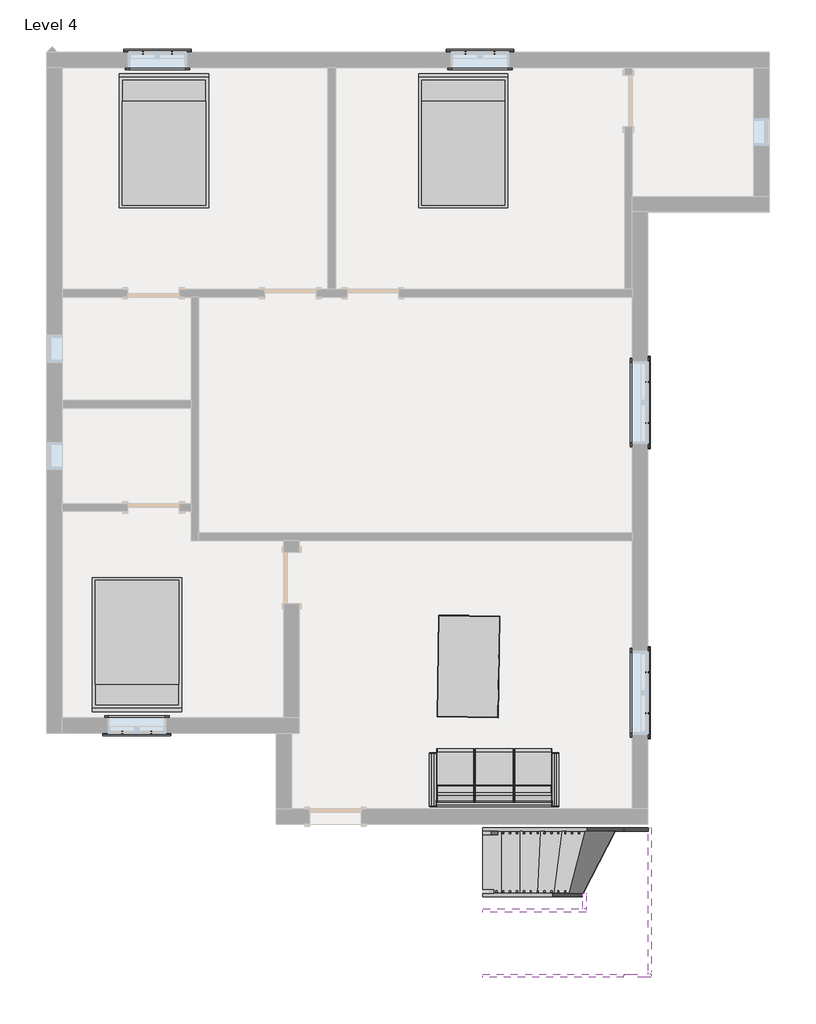
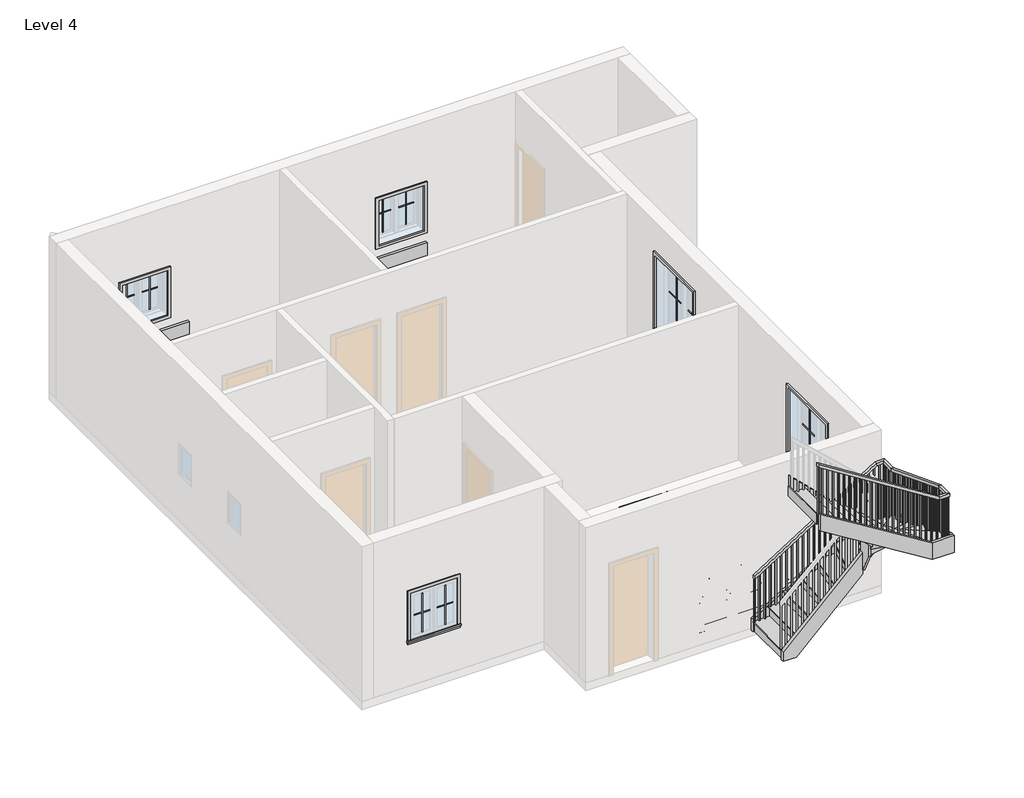
# One storey, part 2 of 2: 20 proxies, 8 members, 5 furniture elements, 1 railing, 1 stair flight.
"""IFC4 building model written with IfcOpenShell, lengths in millimetres."""

from ifc_helpers import new_model, si_unit, frame, origin, place, context, project, spatial, polyline, outline, extrude, faceted_brep, transform, mapped, element, save
from components import muntin_pattern_2x2_muntin_pattern_2x2_b3fe6957, muntin_pattern_2x2_muntin_pattern_2x2_3e0ecaf2, muntin_pattern_2x2_muntin_pattern_2x2_6dad3731, muntin_pattern_2x2_muntin_pattern_2x2_a30a3345, trim_window_exterior_flat_with_sill_41619996, trim_window_exterior_flat_with_sill_92b9b949, trim_window_interior_flat_picture_frame_51c85655, trim_window_interior_flat_picture_frame_3bb882cf, furniture_2fc85b74, furniture_29a9adb8, furniture_57072a26, bed_17739_bed_17739_15c61121, dining_table_14755_dining_table_14755_d89cb775, stair_flight_27d53fa0

model = new_model("IFC4")

# Units and contexts
model_context = context("Model", 3, world=origin())
ifc_project = project(units=[si_unit("LENGTHUNIT", "METRE", prefix="MILLI")], contexts=[model_context])

# Site, building, storey
site = spatial("IfcSite", under=ifc_project)
building = spatial("IfcBuilding", under=site)
storey = spatial("IfcBuildingStorey", under=building, Name="Level 4", Elevation=6400.8)

# Proxies
placement = place(None, origin())
muntin_pattern_2x2_muntin_pattern_2x2_shape = muntin_pattern_2x2_muntin_pattern_2x2_b3fe6957(model_context)
element("IfcBuildingElementProxy", 1, Name="Muntin Pattern_2x2 : Muntin Pattern_2x2", ObjectType="Muntin Pattern_2x2 : Muntin Pattern_2x2", at=placement, inside=storey, context=model_context, shape_type="MappedRepresentation", body=[
    mapped(muntin_pattern_2x2_muntin_pattern_2x2_shape, transform((-4708.0540084, 8034.3685985, 7385.05), x_axis=(1.0, 0.0, 0.0), y_axis=(0.0, 1.0, 0.0), z_axis=(0.0, 0.0, 1.0))),
])
element("IfcBuildingElementProxy", 2, Name="Muntin Pattern_2x2 : Muntin Pattern_2x2", ObjectType="Muntin Pattern_2x2 : Muntin Pattern_2x2", at=placement, inside=storey, context=model_context, shape_type="MappedRepresentation", body=[
    mapped(muntin_pattern_2x2_muntin_pattern_2x2_shape, transform((54.4459916, 8034.3685985, 7385.05), x_axis=(1.0, 0.0, 0.0), y_axis=(0.0, 1.0, 0.0), z_axis=(0.0, 0.0, 1.0))),
])
element("IfcBuildingElementProxy", 3, Name="Muntin Pattern_2x2 : Muntin Pattern_2x2", ObjectType="Muntin Pattern_2x2 : Muntin Pattern_2x2", at=placement, inside=storey, context=model_context, shape_type="MappedRepresentation", body=[
    mapped(muntin_pattern_2x2_muntin_pattern_2x2_shape, transform((-4584.2290084, -2004.9814015, 7385.05), x_axis=(-1.0, 0.0, 0.0), y_axis=(0.0, -1.0, 0.0), z_axis=(0.0, 0.0, 1.0))),
])
muntin_pattern_2x2_muntin_pattern_2x2_2_shape = muntin_pattern_2x2_muntin_pattern_2x2_3e0ecaf2(model_context)
element("IfcBuildingElementProxy", 4, Name="Muntin Pattern_2x2 : Muntin Pattern_2x2", ObjectType="Muntin Pattern_2x2 : Muntin Pattern_2x2", at=placement, inside=storey, context=model_context, shape_type="MappedRepresentation", body=[
    mapped(muntin_pattern_2x2_muntin_pattern_2x2_2_shape, transform((-4279.4290084, 8034.3685985, 7385.05), x_axis=(-1.0, 0.0, 0.0), y_axis=(0.0, -1.0, 0.0), z_axis=(0.0, 0.0, 1.0))),
])
element("IfcBuildingElementProxy", 5, Name="Muntin Pattern_2x2 : Muntin Pattern_2x2", ObjectType="Muntin Pattern_2x2 : Muntin Pattern_2x2", at=placement, inside=storey, context=model_context, shape_type="MappedRepresentation", body=[
    mapped(muntin_pattern_2x2_muntin_pattern_2x2_2_shape, transform((483.0709916, 8034.3685985, 7385.05), x_axis=(-1.0, 0.0, 0.0), y_axis=(0.0, -1.0, 0.0), z_axis=(0.0, 0.0, 1.0))),
])
element("IfcBuildingElementProxy", 6, Name="Muntin Pattern_2x2 : Muntin Pattern_2x2", ObjectType="Muntin Pattern_2x2 : Muntin Pattern_2x2", at=placement, inside=storey, context=model_context, shape_type="MappedRepresentation", body=[
    mapped(muntin_pattern_2x2_muntin_pattern_2x2_2_shape, transform((-5012.8540084, -2004.9814015, 7385.05), x_axis=(1.0, 0.0, 0.0), y_axis=(0.0, 1.0, 0.0), z_axis=(0.0, 0.0, 1.0))),
])
muntin_pattern_2x2_muntin_pattern_2x2_3_shape = muntin_pattern_2x2_muntin_pattern_2x2_6dad3731(model_context)
element("IfcBuildingElementProxy", 7, Name="Muntin Pattern_2x2 : Muntin Pattern_2x2", ObjectType="Muntin Pattern_2x2 : Muntin Pattern_2x2", at=placement, inside=storey, context=model_context, shape_type="MappedRepresentation", body=[
    mapped(muntin_pattern_2x2_muntin_pattern_2x2_3_shape, transform((2735.7334916, -1114.3939015, 7385.05), x_axis=(0.0, -1.0, 0.0), y_axis=(1.0, 0.0, 0.0), z_axis=(0.0, 0.0, 1.0))),
])
element("IfcBuildingElementProxy", 8, Name="Muntin Pattern_2x2 : Muntin Pattern_2x2", ObjectType="Muntin Pattern_2x2 : Muntin Pattern_2x2", at=placement, inside=storey, context=model_context, shape_type="MappedRepresentation", body=[
    mapped(muntin_pattern_2x2_muntin_pattern_2x2_3_shape, transform((2735.7334916, 3171.8560985, 7385.05), x_axis=(0.0, -1.0, 0.0), y_axis=(1.0, 0.0, 0.0), z_axis=(0.0, 0.0, 1.0))),
])
muntin_pattern_2x2_muntin_pattern_2x2_4_shape = muntin_pattern_2x2_muntin_pattern_2x2_a30a3345(model_context)
element("IfcBuildingElementProxy", 9, Name="Muntin Pattern_2x2 : Muntin Pattern_2x2", ObjectType="Muntin Pattern_2x2 : Muntin Pattern_2x2", at=placement, inside=storey, context=model_context, shape_type="MappedRepresentation", body=[
    mapped(muntin_pattern_2x2_muntin_pattern_2x2_4_shape, transform((2735.7334916, -1720.8189015, 7385.05), x_axis=(0.0, 1.0, 0.0), y_axis=(-1.0, 0.0, 0.0), z_axis=(0.0, 0.0, 1.0))),
])
element("IfcBuildingElementProxy", 10, Name="Muntin Pattern_2x2 : Muntin Pattern_2x2", ObjectType="Muntin Pattern_2x2 : Muntin Pattern_2x2", at=placement, inside=storey, context=model_context, shape_type="MappedRepresentation", body=[
    mapped(muntin_pattern_2x2_muntin_pattern_2x2_4_shape, transform((2735.7334916, 2565.4310985, 7385.05), x_axis=(0.0, 1.0, 0.0), y_axis=(-1.0, 0.0, 0.0), z_axis=(0.0, 0.0, 1.0))),
])
trim_window_exterior_flat_with_sill_shape = trim_window_exterior_flat_with_sill_41619996(model_context)
element("IfcBuildingElementProxy", 11, Name="Trim-Window-Exterior-Flat : with Sill", ObjectType="Trim-Window-Exterior-Flat : with Sill", at=placement, inside=storey, context=model_context, shape_type="MappedRepresentation", body=[
    mapped(trim_window_exterior_flat_with_sill_shape, transform((-4493.7415084, 8043.8935985, 8229.6), x_axis=(-1.0, 0.0, 0.0), y_axis=(0.0, 0.0, 1.0), z_axis=(0.0, 1.0, 0.0))),
])
element("IfcBuildingElementProxy", 12, Name="Trim-Window-Exterior-Flat : with Sill", ObjectType="Trim-Window-Exterior-Flat : with Sill", at=placement, inside=storey, context=model_context, shape_type="MappedRepresentation", body=[
    mapped(trim_window_exterior_flat_with_sill_shape, transform((268.7584916, 8043.8935985, 8229.6), x_axis=(-1.0, 0.0, 0.0), y_axis=(0.0, 0.0, 1.0), z_axis=(0.0, 1.0, 0.0))),
])
element("IfcBuildingElementProxy", 13, Name="Trim-Window-Exterior-Flat : with Sill", ObjectType="Trim-Window-Exterior-Flat : with Sill", at=placement, inside=storey, context=model_context, shape_type="MappedRepresentation", body=[
    mapped(trim_window_exterior_flat_with_sill_shape, transform((-4798.5415084, -2014.5064015, 8229.6), x_axis=(1.0, 0.0, 0.0), y_axis=(0.0, 0.0, 1.0), z_axis=(0.0, -1.0, 0.0))),
])
trim_window_exterior_flat_with_sill_2_shape = trim_window_exterior_flat_with_sill_92b9b949(model_context)
element("IfcBuildingElementProxy", 14, Name="Trim-Window-Exterior-Flat : with Sill", ObjectType="Trim-Window-Exterior-Flat : with Sill", at=placement, inside=storey, context=model_context, shape_type="MappedRepresentation", body=[
    mapped(trim_window_exterior_flat_with_sill_2_shape, transform((2745.2584916, -1417.6064015, 8839.2), x_axis=(0.0, 1.0, 0.0), y_axis=(0.0, 0.0, 1.0), z_axis=(1.0, 0.0, 0.0))),
])
element("IfcBuildingElementProxy", 15, Name="Trim-Window-Exterior-Flat : with Sill", ObjectType="Trim-Window-Exterior-Flat : with Sill", at=placement, inside=storey, context=model_context, shape_type="MappedRepresentation", body=[
    mapped(trim_window_exterior_flat_with_sill_2_shape, transform((2745.2584916, 2868.6435985, 8839.2), x_axis=(0.0, 1.0, 0.0), y_axis=(0.0, 0.0, 1.0), z_axis=(1.0, 0.0, 0.0))),
])
trim_window_interior_flat_picture_frame_shape = trim_window_interior_flat_picture_frame_51c85655(model_context)
element("IfcBuildingElementProxy", 16, Name="Trim-Window-Interior-Flat : Picture Frame", ObjectType="Trim-Window-Interior-Flat : Picture Frame", at=placement, inside=storey, context=model_context, shape_type="MappedRepresentation", body=[
    mapped(trim_window_interior_flat_picture_frame_shape, transform((-4493.7415084, 7815.2935985, 8229.6), x_axis=(1.0, 0.0, 0.0), y_axis=(0.0, 0.0, 1.0), z_axis=(0.0, -1.0, 0.0))),
])
element("IfcBuildingElementProxy", 17, Name="Trim-Window-Interior-Flat : Picture Frame", ObjectType="Trim-Window-Interior-Flat : Picture Frame", at=placement, inside=storey, context=model_context, shape_type="MappedRepresentation", body=[
    mapped(trim_window_interior_flat_picture_frame_shape, transform((268.7584916, 7815.2935985, 8229.6), x_axis=(1.0, 0.0, 0.0), y_axis=(0.0, 0.0, 1.0), z_axis=(0.0, -1.0, 0.0))),
])
element("IfcBuildingElementProxy", 18, Name="Trim-Window-Interior-Flat : Picture Frame", ObjectType="Trim-Window-Interior-Flat : Picture Frame", at=placement, inside=storey, context=model_context, shape_type="MappedRepresentation", body=[
    mapped(trim_window_interior_flat_picture_frame_shape, transform((-4798.5415084, -1785.9064015, 8229.6), x_axis=(-1.0, 0.0, 0.0), y_axis=(0.0, 0.0, 1.0), z_axis=(0.0, 1.0, 0.0))),
])
trim_window_interior_flat_picture_frame_2_shape = trim_window_interior_flat_picture_frame_3bb882cf(model_context)
element("IfcBuildingElementProxy", 19, Name="Trim-Window-Interior-Flat : Picture Frame", ObjectType="Trim-Window-Interior-Flat : Picture Frame", at=placement, inside=storey, context=model_context, shape_type="MappedRepresentation", body=[
    mapped(trim_window_interior_flat_picture_frame_2_shape, transform((2516.6584916, -1417.6064015, 8839.2), x_axis=(0.0, -1.0, 0.0), y_axis=(0.0, 0.0, 1.0), z_axis=(-1.0, 0.0, 0.0))),
])
element("IfcBuildingElementProxy", 20, Name="Trim-Window-Interior-Flat : Picture Frame", ObjectType="Trim-Window-Interior-Flat : Picture Frame", at=placement, inside=storey, context=model_context, shape_type="MappedRepresentation", body=[
    mapped(trim_window_interior_flat_picture_frame_2_shape, transform((2516.6584916, 2868.6435985, 8839.2), x_axis=(0.0, -1.0, 0.0), y_axis=(0.0, 0.0, 1.0), z_axis=(-1.0, 0.0, 0.0))),
])

# Furniture
furniture_shape = furniture_2fc85b74(model_context)
furniture_2_shape = furniture_29a9adb8(model_context)
furniture_3_shape = furniture_57072a26(model_context)
element("IfcFurniture", 21, at=placement, inside=storey, context=model_context, shape_type="MappedRepresentation", body=[
    mapped(furniture_shape, transform((477.9947981, -2301.7922014, 6400.8), x_axis=(-1.0, 0.0, 0.0), y_axis=(0.0, -1.0, 0.0), z_axis=(0.0, 0.0, 1.0))),
    mapped(furniture_2_shape, transform((477.9947981, -2301.7922014, 6400.8), x_axis=(-1.0, 0.0, 0.0), y_axis=(0.0, -1.0, 0.0), z_axis=(0.0, 0.0, 1.0))),
    mapped(furniture_3_shape, transform((477.9947981, -2301.7922014, 6400.8), x_axis=(-1.0, 0.0, 0.0), y_axis=(0.0, -1.0, 0.0), z_axis=(0.0, 0.0, 1.0))),
])
bed_17739_bed_17739_shape = bed_17739_bed_17739_15c61121(model_context)
element("IfcFurniture", 22, ObjectType="Bed_17739 : Bed_17739", at=placement, inside=storey, context=model_context, shape_type="MappedRepresentation", body=[
    mapped(bed_17739_bed_17739_shape, transform((-4398.4915084, 6710.3935985, 6400.8), x_axis=(1.0, 0.0, 0.0), y_axis=(0.0, 1.0, 0.0), z_axis=(0.0, 0.0, 1.0))),
])
element("IfcFurniture", 23, ObjectType="Bed_17739 : Bed_17739", at=placement, inside=storey, context=model_context, shape_type="MappedRepresentation", body=[
    mapped(bed_17739_bed_17739_shape, transform((21.1084916, 6710.3935985, 6400.8), x_axis=(1.0, 0.0, 0.0), y_axis=(0.0, 1.0, 0.0), z_axis=(0.0, 0.0, 1.0))),
])
element("IfcFurniture", 24, ObjectType="Bed_17739 : Bed_17739", at=placement, inside=storey, context=model_context, shape_type="MappedRepresentation", body=[
    mapped(bed_17739_bed_17739_shape, transform((-4798.5415084, -681.0064015, 6400.8), x_axis=(-1.0, 0.0, 0.0), y_axis=(0.0, -1.0, 0.0), z_axis=(0.0, 0.0, 1.0))),
])
dining_table_14755_dining_table_14755_shape = dining_table_14755_dining_table_14755_d89cb775(model_context)
element("IfcFurniture", 25, ObjectType="Dining_table_14755 : Dining_table_14755", at=placement, inside=storey, context=model_context, shape_type="MappedRepresentation", body=[
    mapped(dining_table_14755_dining_table_14755_shape, transform((535.647979, -1785.9064015, 6400.8), x_axis=(0.016088397262737867, 0.9998705733611308, 0.0), y_axis=(-0.9998705733611308, 0.016088397262737867, 0.0), z_axis=(0.0, 0.0, 1.0))),
])

# Members
element("IfcMember", 26, ObjectType="Stringer - 2\" Width", at=placement, inside=storey, context=model_context, shape_type="SweptSolid", body=[
    extrude(outline(polyline([(6644.4922047, 306.9570026), (6400.8, 306.9570026), (6400.8, 492.4029437), (7577.0227917, 2394.3741942), (7935.3990341, 2394.3741942), (6644.4922047, 306.9570026)])), frame((0.0, -3462.3064015, 0.0), z_axis=(0.0, 1.0, 0.0), x_axis=(0.0, 0.0, 1.0)), (0.0, 0.0, 1.0), 50.8),
])
element("IfcMember", 27, ObjectType="Stringer - 2\" Width", at=placement, inside=storey, context=model_context, shape_type="SweptSolid", body=[
    extrude(outline(polyline([(2394.3741942, -3462.3064015), (2394.3741942, -3411.5064015), (2749.0886944, -3411.5064015), (2749.0886944, -3462.3064015), (2394.3741942, -3462.3064015)])), frame((0.0, 0.0, 7577.0227917), z_axis=(0.0, 0.0, 1.0), x_axis=(1.0, 0.0, 0.0)), (0.0, 0.0, 1.0), 358.3762424),
])
element("IfcMember", 28, ObjectType="Stringer - 2\" Width", at=placement, inside=storey, context=model_context, shape_type="SweptSolid", body=[
    extrude(outline(polyline([(-3411.5064015, 7915.8385252), (-3411.5064015, 7630.5990341), (-3601.4476233, 7630.5990341), (-5570.5064015, 8388.7839126), (-5570.5064015, 8729.4251697), (-5524.4474131, 8729.4251697), (-3411.5064015, 7915.8385252)])), frame((2749.0886944, 0.0, 0.0), z_axis=(1.0, 0.0, 0.0), x_axis=(0.0, 1.0, 0.0)), (0.0, 0.0, 1.0), 50.8),
])
element("IfcMember", 29, ObjectType="Stringer - 2\" Width", at=placement, inside=storey, context=model_context, shape_type="SweptSolid", body=[
    extrude(outline(polyline([(2799.8886944, -5570.5064015), (2799.8886944, -5621.3064015), (2394.3741942, -5621.3064015), (2394.3741942, -5570.5064015), (2799.8886944, -5570.5064015)])), frame((0.0, 0.0, 8402.8105246), z_axis=(0.0, 0.0, 1.0), x_axis=(1.0, 0.0, 0.0)), (0.0, 0.0, 1.0), 326.614645),
])
element("IfcMember", 30, ObjectType="Stringer - 2\" Width", at=placement, inside=storey, context=model_context, shape_type="SweptSolid", body=[
    extrude(outline(polyline([(8402.8105246, 2394.3741942), (8729.4251697, 2394.3741942), (10020.3319991, 306.9570026), (9693.7173541, 306.9570026), (8402.8105246, 2394.3741942)])), frame((0.0, -5621.3064015, 0.0), z_axis=(0.0, 1.0, 0.0), x_axis=(0.0, 0.0, 1.0)), (0.0, 0.0, 1.0), 50.8),
])
element("IfcMember", 31, ObjectType="Stringer - 2\" Width", at=placement, inside=storey, context=model_context, shape_type="SweptSolid", body=[
    extrude(outline(polyline([(6586.349344, 306.9570026), (6400.8, 306.9570026), (6400.8, 553.146333), (7605.0088874, 1783.8886944), (8031.4399862, 1783.8886944), (6586.349344, 306.9570026)])), frame((0.0, -4427.5064015, 0.0), z_axis=(0.0, 1.0, 0.0), x_axis=(0.0, 0.0, 1.0)), (0.0, 0.0, 1.0), 50.8),
])
element("IfcMember", 32, ObjectType="Stringer - 2\" Width", at=placement, inside=storey, context=model_context, shape_type="SweptSolid", body=[
    extrude(outline(polyline([(-4376.7064015, 8276.0734955), (-4376.7064015, 7654.7136944), (-4412.6455235, 7654.7136944), (-4605.3064015, 8049.5203552), (-4605.3064015, 8686.3067712), (-4576.8952811, 8686.3067712), (-4376.7064015, 8276.0734955)])), frame((1783.8886944, 0.0, 0.0), z_axis=(1.0, 0.0, 0.0), x_axis=(0.0, 1.0, 0.0)), (0.0, 0.0, 1.0), 50.8),
])
element("IfcMember", 33, ObjectType="Stringer - 2\" Width", at=placement, inside=storey, context=model_context, shape_type="SweptSolid", body=[
    extrude(outline(polyline([(8259.8756724, 1834.6886944), (8686.3067712, 1834.6886944), (10181.1022205, 306.9570026), (9754.6711216, 306.9570026), (8259.8756724, 1834.6886944)])), frame((0.0, -4656.1064015, 0.0), z_axis=(0.0, 1.0, 0.0), x_axis=(0.0, 0.0, 1.0)), (0.0, 0.0, 1.0), 50.8),
])

# Railing
element("IfcRailing", 34, ObjectType="Handrail - Rectangular", at=placement, inside=storey, context=model_context, shape_type="SolidModel", body=[
    faceted_brep([(306.9570026, -3462.3064015, 7518.4), (306.9570026, -3462.3064015, 7458.2440152), (306.9570026, -3513.1064015, 7458.2440152), (306.9570026, -3513.1064015, 7518.4), (2564.6820646, -3462.3064015, 8950.3487041), (2579.4334598, -3462.3064015, 8899.5487041), (2579.4334598, -3513.1064015, 8899.5487041), (2564.6820646, -3513.1064015, 8950.3487041), (2749.0886944, -3462.3064015, 8950.3487041), (2749.0886944, -3462.3064015, 8899.5487041), (2698.2886944, -3513.1064015, 8899.5487041), (2698.2886944, -3513.1064015, 8950.3487041), (2749.0886944, -3749.6182836, 8950.3487041), (2749.0886944, -3759.0606416, 8899.5487041), (2698.2886944, -3759.0606416, 8899.5487041), (2698.2886944, -3749.6182836, 8950.3487041), (2749.0886944, -5283.1945194, 9540.8512959), (2749.0886944, -5292.6368774, 9490.0512959), (2698.2886944, -5292.6368774, 9490.0512959), (2698.2886944, -5283.1945194, 9540.8512959), (2749.0886944, -5570.5064015, 9540.8512959), (2749.0886944, -5570.5064015, 9490.0512959), (2698.2886944, -5519.7064015, 9490.0512959), (2698.2886944, -5519.7064015, 9540.8512959), (2564.6820646, -5570.5064015, 9540.8512959), (2549.9306694, -5570.5064015, 9490.0512959), (2549.9306694, -5519.7064015, 9490.0512959), (2564.6820646, -5519.7064015, 9540.8512959), (306.9570026, -5570.5064015, 10972.8), (306.9570026, -5519.7064015, 10972.8), (306.9570026, -5519.7064015, 10912.6440152), (306.9570026, -5570.5064015, 10912.6440152)], [[[0, 1, 2, 3]], [[1, 0, 4, 5]], [[2, 1, 5, 6]], [[3, 2, 6, 7]], [[0, 3, 7, 4]], [[5, 4, 8, 9]], [[6, 5, 9, 10]], [[7, 6, 10, 11]], [[4, 7, 11, 8]], [[9, 8, 12, 13]], [[10, 9, 13, 14]], [[11, 10, 14, 15]], [[8, 11, 15, 12]], [[13, 12, 16, 17]], [[14, 13, 17, 18]], [[15, 14, 18, 19]], [[12, 15, 19, 16]], [[17, 16, 20, 21]], [[18, 17, 21, 22]], [[19, 18, 22, 23]], [[16, 19, 23, 20]], [[21, 20, 24, 25]], [[22, 21, 25, 26]], [[23, 22, 26, 27]], [[20, 23, 27, 24]], [[28, 29, 30, 31]], [[25, 24, 28, 31]], [[26, 25, 31, 30]], [[27, 26, 30, 29]], [[24, 27, 29, 28]]]),
    extrude(outline(polyline([(10867.9889893, 377.3636944), (9855.2, 377.3636944), (9855.2, 396.4136944), (10855.90664, 396.4136944), (10867.9889893, 377.3636944)])), frame((0.0, -5554.6314015, 0.0), z_axis=(0.0, 1.0, 0.0), x_axis=(0.0, 0.0, 1.0)), (0.0, 0.0, 1.0), 19.05),
    extrude(outline(polyline([(10803.5497931, 478.9636944), (9855.2, 478.9636944), (9855.2, 498.0136944), (10791.4674438, 498.0136944), (10803.5497931, 478.9636944)])), frame((0.0, -5554.6314015, 0.0), z_axis=(0.0, 1.0, 0.0), x_axis=(0.0, 0.0, 1.0)), (0.0, 0.0, 1.0), 19.05),
    extrude(outline(polyline([(10739.1105968, 580.5636944), (9652.0, 580.5636944), (9652.0, 599.6136944), (10727.0282475, 599.6136944), (10739.1105968, 580.5636944)])), frame((0.0, -5554.6314015, 0.0), z_axis=(0.0, 1.0, 0.0), x_axis=(0.0, 0.0, 1.0)), (0.0, 0.0, 1.0), 19.05),
    extrude(outline(polyline([(10674.6714006, 682.1636944), (9652.0, 682.1636944), (9652.0, 701.2136944), (10662.5890513, 701.2136944), (10674.6714006, 682.1636944)])), frame((0.0, -5554.6314015, 0.0), z_axis=(0.0, 1.0, 0.0), x_axis=(0.0, 0.0, 1.0)), (0.0, 0.0, 1.0), 19.05),
    extrude(outline(polyline([(10610.2322043, 783.7636944), (9652.0, 783.7636944), (9652.0, 802.8136944), (10598.149855, 802.8136944), (10610.2322043, 783.7636944)])), frame((0.0, -5554.6314015, 0.0), z_axis=(0.0, 1.0, 0.0), x_axis=(0.0, 0.0, 1.0)), (0.0, 0.0, 1.0), 19.05),
    extrude(outline(polyline([(10545.7930081, 885.3636944), (9448.8, 885.3636944), (9448.8, 904.4136944), (10533.7106588, 904.4136944), (10545.7930081, 885.3636944)])), frame((0.0, -5554.6314015, 0.0), z_axis=(0.0, 1.0, 0.0), x_axis=(0.0, 0.0, 1.0)), (0.0, 0.0, 1.0), 19.05),
    extrude(outline(polyline([(10481.3538119, 986.9636944), (9448.8, 986.9636944), (9448.8, 1006.0136944), (10469.2714626, 1006.0136944), (10481.3538119, 986.9636944)])), frame((0.0, -5554.6314015, 0.0), z_axis=(0.0, 1.0, 0.0), x_axis=(0.0, 0.0, 1.0)), (0.0, 0.0, 1.0), 19.05),
    extrude(outline(polyline([(10416.9146156, 1088.5636944), (9448.8, 1088.5636944), (9448.8, 1107.6136944), (10404.8322663, 1107.6136944), (10416.9146156, 1088.5636944)])), frame((0.0, -5554.6314015, 0.0), z_axis=(0.0, 1.0, 0.0), x_axis=(0.0, 0.0, 1.0)), (0.0, 0.0, 1.0), 19.05),
    extrude(outline(polyline([(10352.4754194, 1190.1636944), (9245.6, 1190.1636944), (9245.6, 1209.2136944), (10340.3930701, 1209.2136944), (10352.4754194, 1190.1636944)])), frame((0.0, -5554.6314015, 0.0), z_axis=(0.0, 1.0, 0.0), x_axis=(0.0, 0.0, 1.0)), (0.0, 0.0, 1.0), 19.05),
    extrude(outline(polyline([(10288.0362231, 1291.7636944), (9245.6, 1291.7636944), (9245.6, 1310.8136944), (10275.9538738, 1310.8136944), (10288.0362231, 1291.7636944)])), frame((0.0, -5554.6314015, 0.0), z_axis=(0.0, 1.0, 0.0), x_axis=(0.0, 0.0, 1.0)), (0.0, 0.0, 1.0), 19.05),
    extrude(outline(polyline([(10223.5970269, 1393.3636944), (9245.6, 1393.3636944), (9245.6, 1412.4136944), (10211.5146776, 1412.4136944), (10223.5970269, 1393.3636944)])), frame((0.0, -5554.6314015, 0.0), z_axis=(0.0, 1.0, 0.0), x_axis=(0.0, 0.0, 1.0)), (0.0, 0.0, 1.0), 19.05),
    extrude(outline(polyline([(10159.1578306, 1494.9636944), (9042.4, 1494.9636944), (9042.4, 1514.0136944), (10147.0754813, 1514.0136944), (10159.1578306, 1494.9636944)])), frame((0.0, -5554.6314015, 0.0), z_axis=(0.0, 1.0, 0.0), x_axis=(0.0, 0.0, 1.0)), (0.0, 0.0, 1.0), 19.05),
    extrude(outline(polyline([(10094.7186344, 1596.5636944), (9042.4, 1596.5636944), (9042.4, 1615.6136944), (10082.6362851, 1615.6136944), (10094.7186344, 1596.5636944)])), frame((0.0, -5554.6314015, 0.0), z_axis=(0.0, 1.0, 0.0), x_axis=(0.0, 0.0, 1.0)), (0.0, 0.0, 1.0), 19.05),
    extrude(outline(polyline([(10030.2794382, 1698.1636944), (9042.4, 1698.1636944), (9042.4, 1717.2136944), (10018.1970889, 1717.2136944), (10030.2794382, 1698.1636944)])), frame((0.0, -5554.6314015, 0.0), z_axis=(0.0, 1.0, 0.0), x_axis=(0.0, 0.0, 1.0)), (0.0, 0.0, 1.0), 19.05),
    extrude(outline(polyline([(9965.8402419, 1799.7636944), (9042.4, 1799.7636944), (9042.4, 1818.8136944), (9953.7578926, 1818.8136944), (9965.8402419, 1799.7636944)])), frame((0.0, -5554.6314015, 0.0), z_axis=(0.0, 1.0, 0.0), x_axis=(0.0, 0.0, 1.0)), (0.0, 0.0, 1.0), 19.05),
    extrude(outline(polyline([(9901.4010457, 1901.3636944), (8839.2, 1901.3636944), (8839.2, 1920.4136944), (9889.3186964, 1920.4136944), (9901.4010457, 1901.3636944)])), frame((0.0, -5554.6314015, 0.0), z_axis=(0.0, 1.0, 0.0), x_axis=(0.0, 0.0, 1.0)), (0.0, 0.0, 1.0), 19.05),
    extrude(outline(polyline([(9836.9618494, 2002.9636944), (8839.2, 2002.9636944), (8839.2, 2022.0136944), (9824.8795001, 2022.0136944), (9836.9618494, 2002.9636944)])), frame((0.0, -5554.6314015, 0.0), z_axis=(0.0, 1.0, 0.0), x_axis=(0.0, 0.0, 1.0)), (0.0, 0.0, 1.0), 19.05),
    extrude(outline(polyline([(9772.5226532, 2104.5636944), (8839.2, 2104.5636944), (8839.2, 2123.6136944), (9760.4403039, 2123.6136944), (9772.5226532, 2104.5636944)])), frame((0.0, -5554.6314015, 0.0), z_axis=(0.0, 1.0, 0.0), x_axis=(0.0, 0.0, 1.0)), (0.0, 0.0, 1.0), 19.05),
    extrude(outline(polyline([(9708.0834569, 2206.1636944), (8839.2, 2206.1636944), (8839.2, 2225.2136944), (9696.0011076, 2225.2136944), (9708.0834569, 2206.1636944)])), frame((0.0, -5554.6314015, 0.0), z_axis=(0.0, 1.0, 0.0), x_axis=(0.0, 0.0, 1.0)), (0.0, 0.0, 1.0), 19.05),
    extrude(outline(polyline([(9643.6442607, 2307.7636944), (8636.0, 2307.7636944), (8636.0, 2326.8136944), (9631.5619114, 2326.8136944), (9643.6442607, 2307.7636944)])), frame((0.0, -5554.6314015, 0.0), z_axis=(0.0, 1.0, 0.0), x_axis=(0.0, 0.0, 1.0)), (0.0, 0.0, 1.0), 19.05),
    extrude(outline(polyline([(9579.2050645, 2409.3636944), (8636.0, 2409.3636944), (8636.0, 2428.4136944), (9567.1227152, 2428.4136944), (9579.2050645, 2409.3636944)])), frame((0.0, -5554.6314015, 0.0), z_axis=(0.0, 1.0, 0.0), x_axis=(0.0, 0.0, 1.0)), (0.0, 0.0, 1.0), 19.05),
    extrude(outline(polyline([(9514.7658682, 2510.9636944), (8636.0, 2510.9636944), (8636.0, 2530.0136944), (9502.6835189, 2530.0136944), (9514.7658682, 2510.9636944)])), frame((0.0, -5554.6314015, 0.0), z_axis=(0.0, 1.0, 0.0), x_axis=(0.0, 0.0, 1.0)), (0.0, 0.0, 1.0), 19.05),
    extrude(outline(polyline([(2631.6136944, -5554.6314015), (2612.5636944, -5554.6314015), (2612.5636944, -5535.5814015), (2631.6136944, -5535.5814015), (2631.6136944, -5554.6314015)])), frame((0.0, 0.0, 8636.0), z_axis=(0.0, 0.0, 1.0), x_axis=(1.0, 0.0, 0.0)), (0.0, 0.0, 1.0), 854.0512959),
    extrude(outline(polyline([(2733.2136944, -5510.1814015), (2733.2136944, -5529.2314015), (2714.1636944, -5529.2314015), (2714.1636944, -5510.1814015), (2733.2136944, -5510.1814015)])), frame((0.0, 0.0, 8636.0), z_axis=(0.0, 0.0, 1.0), x_axis=(1.0, 0.0, 0.0)), (0.0, 0.0, 1.0), 854.0512959),
    extrude(outline(polyline([(2733.2136944, -5408.5814015), (2733.2136944, -5427.6314015), (2714.1636944, -5427.6314015), (2714.1636944, -5408.5814015), (2733.2136944, -5408.5814015)])), frame((0.0, 0.0, 8636.0), z_axis=(0.0, 0.0, 1.0), x_axis=(1.0, 0.0, 0.0)), (0.0, 0.0, 1.0), 854.0512959),
    extrude(outline(polyline([(2733.2136944, -5306.9814015), (2733.2136944, -5326.0314015), (2714.1636944, -5326.0314015), (2714.1636944, -5306.9814015), (2733.2136944, -5306.9814015)])), frame((0.0, 0.0, 8636.0), z_axis=(0.0, 0.0, 1.0), x_axis=(1.0, 0.0, 0.0)), (0.0, 0.0, 1.0), 854.0512959),
    extrude(outline(polyline([(-5205.3814015, 9456.4536283), (-5205.3814015, 8432.8), (-5224.4314015, 8432.8), (-5224.4314015, 9463.7888191), (-5205.3814015, 9456.4536283)])), frame((2714.1636944, 0.0, 0.0), z_axis=(1.0, 0.0, 0.0), x_axis=(0.0, 1.0, 0.0)), (0.0, 0.0, 1.0), 19.05),
    extrude(outline(polyline([(-5103.7814015, 9417.3326104), (-5103.7814015, 8432.8), (-5122.8314015, 8432.8), (-5122.8314015, 9424.6678013), (-5103.7814015, 9417.3326104)])), frame((2714.1636944, 0.0, 0.0), z_axis=(1.0, 0.0, 0.0), x_axis=(0.0, 1.0, 0.0)), (0.0, 0.0, 1.0), 19.05),
    extrude(outline(polyline([(-5002.1814015, 9378.2115925), (-5002.1814015, 8432.8), (-5021.2314015, 8432.8), (-5021.2314015, 9385.5467834), (-5002.1814015, 9378.2115925)])), frame((2714.1636944, 0.0, 0.0), z_axis=(1.0, 0.0, 0.0), x_axis=(0.0, 1.0, 0.0)), (0.0, 0.0, 1.0), 19.05),
    extrude(outline(polyline([(-4900.5814015, 9339.0905747), (-4900.5814015, 8432.8), (-4919.6314015, 8432.8), (-4919.6314015, 9346.4257655), (-4900.5814015, 9339.0905747)])), frame((2714.1636944, 0.0, 0.0), z_axis=(1.0, 0.0, 0.0), x_axis=(0.0, 1.0, 0.0)), (0.0, 0.0, 1.0), 19.05),
    extrude(outline(polyline([(-4798.9814015, 9299.9695568), (-4798.9814015, 8432.8), (-4818.0314015, 8432.8), (-4818.0314015, 9307.3047476), (-4798.9814015, 9299.9695568)])), frame((2714.1636944, 0.0, 0.0), z_axis=(1.0, 0.0, 0.0), x_axis=(0.0, 1.0, 0.0)), (0.0, 0.0, 1.0), 19.05),
    extrude(outline(polyline([(-4697.3814015, 9260.8485389), (-4697.3814015, 8229.6), (-4716.4314015, 8229.6), (-4716.4314015, 9268.1837298), (-4697.3814015, 9260.8485389)])), frame((2714.1636944, 0.0, 0.0), z_axis=(1.0, 0.0, 0.0), x_axis=(0.0, 1.0, 0.0)), (0.0, 0.0, 1.0), 19.05),
    extrude(outline(polyline([(-4595.7814015, 9221.727521), (-4595.7814015, 8229.6), (-4614.8314015, 8229.6), (-4614.8314015, 9229.0627119), (-4595.7814015, 9221.727521)])), frame((2714.1636944, 0.0, 0.0), z_axis=(1.0, 0.0, 0.0), x_axis=(0.0, 1.0, 0.0)), (0.0, 0.0, 1.0), 19.05),
    extrude(outline(polyline([(-4494.1814015, 9182.6065032), (-4494.1814015, 8229.6), (-4513.2314015, 8229.6), (-4513.2314015, 9189.941694), (-4494.1814015, 9182.6065032)])), frame((2714.1636944, 0.0, 0.0), z_axis=(1.0, 0.0, 0.0), x_axis=(0.0, 1.0, 0.0)), (0.0, 0.0, 1.0), 19.05),
    extrude(outline(polyline([(-4392.5814015, 9143.4854853), (-4392.5814015, 8229.6), (-4411.6314015, 8229.6), (-4411.6314015, 9150.8206761), (-4392.5814015, 9143.4854853)])), frame((2714.1636944, 0.0, 0.0), z_axis=(1.0, 0.0, 0.0), x_axis=(0.0, 1.0, 0.0)), (0.0, 0.0, 1.0), 19.05),
    extrude(outline(polyline([(-4290.9814015, 9104.3644674), (-4290.9814015, 8229.6), (-4310.0314015, 8229.6), (-4310.0314015, 9111.6996583), (-4290.9814015, 9104.3644674)])), frame((2714.1636944, 0.0, 0.0), z_axis=(1.0, 0.0, 0.0), x_axis=(0.0, 1.0, 0.0)), (0.0, 0.0, 1.0), 19.05),
    extrude(outline(polyline([(-4189.3814015, 9065.2434495), (-4189.3814015, 8026.4), (-4208.4314015, 8026.4), (-4208.4314015, 9072.5786404), (-4189.3814015, 9065.2434495)])), frame((2714.1636944, 0.0, 0.0), z_axis=(1.0, 0.0, 0.0), x_axis=(0.0, 1.0, 0.0)), (0.0, 0.0, 1.0), 19.05),
    extrude(outline(polyline([(-4087.7814015, 9026.1224317), (-4087.7814015, 8026.4), (-4106.8314015, 8026.4), (-4106.8314015, 9033.4576225), (-4087.7814015, 9026.1224317)])), frame((2714.1636944, 0.0, 0.0), z_axis=(1.0, 0.0, 0.0), x_axis=(0.0, 1.0, 0.0)), (0.0, 0.0, 1.0), 19.05),
    extrude(outline(polyline([(-3986.1814015, 8987.0014138), (-3986.1814015, 8026.4), (-4005.2314015, 8026.4), (-4005.2314015, 8994.3366047), (-3986.1814015, 8987.0014138)])), frame((2714.1636944, 0.0, 0.0), z_axis=(1.0, 0.0, 0.0), x_axis=(0.0, 1.0, 0.0)), (0.0, 0.0, 1.0), 19.05),
    extrude(outline(polyline([(-3884.5814015, 8947.8803959), (-3884.5814015, 8026.4), (-3903.6314015, 8026.4), (-3903.6314015, 8955.2155868), (-3884.5814015, 8947.8803959)])), frame((2714.1636944, 0.0, 0.0), z_axis=(1.0, 0.0, 0.0), x_axis=(0.0, 1.0, 0.0)), (0.0, 0.0, 1.0), 19.05),
    extrude(outline(polyline([(-3782.9814015, 8908.7593781), (-3782.9814015, 8026.4), (-3802.0314015, 8026.4), (-3802.0314015, 8916.0945689), (-3782.9814015, 8908.7593781)])), frame((2714.1636944, 0.0, 0.0), z_axis=(1.0, 0.0, 0.0), x_axis=(0.0, 1.0, 0.0)), (0.0, 0.0, 1.0), 19.05),
    extrude(outline(polyline([(2733.2136944, -3681.3814015), (2733.2136944, -3700.4314015), (2714.1636944, -3700.4314015), (2714.1636944, -3681.3814015), (2733.2136944, -3681.3814015)])), frame((0.0, 0.0, 7823.2), z_axis=(0.0, 0.0, 1.0), x_axis=(1.0, 0.0, 0.0)), (0.0, 0.0, 1.0), 1076.3487041),
    extrude(outline(polyline([(2733.2136944, -3579.7814015), (2733.2136944, -3598.8314015), (2714.1636944, -3598.8314015), (2714.1636944, -3579.7814015), (2733.2136944, -3579.7814015)])), frame((0.0, 0.0, 7823.2), z_axis=(0.0, 0.0, 1.0), x_axis=(1.0, 0.0, 0.0)), (0.0, 0.0, 1.0), 1076.3487041),
    extrude(outline(polyline([(2634.2320026, -3478.1814015), (2653.2820026, -3478.1814015), (2653.2820026, -3497.2314015), (2634.2320026, -3497.2314015), (2634.2320026, -3478.1814015)])), frame((0.0, 0.0, 7823.2), z_axis=(0.0, 0.0, 1.0), x_axis=(1.0, 0.0, 0.0)), (0.0, 0.0, 1.0), 1076.3487041),
    extrude(outline(polyline([(8869.8651579, 2532.6320026), (7823.2, 2532.6320026), (7823.2, 2551.6820026), (8881.9475072, 2551.6820026), (8869.8651579, 2532.6320026)])), frame((0.0, -3497.2314015, 0.0), z_axis=(0.0, 1.0, 0.0), x_axis=(0.0, 0.0, 1.0)), (0.0, 0.0, 1.0), 19.05),
    extrude(outline(polyline([(8805.4259617, 2431.0320026), (7823.2, 2431.0320026), (7823.2, 2450.0820026), (8817.508311, 2450.0820026), (8805.4259617, 2431.0320026)])), frame((0.0, -3497.2314015, 0.0), z_axis=(0.0, 1.0, 0.0), x_axis=(0.0, 0.0, 1.0)), (0.0, 0.0, 1.0), 19.05),
    extrude(outline(polyline([(8740.9867654, 2329.4320026), (7823.2, 2329.4320026), (7823.2, 2348.4820026), (8753.0691147, 2348.4820026), (8740.9867654, 2329.4320026)])), frame((0.0, -3497.2314015, 0.0), z_axis=(0.0, 1.0, 0.0), x_axis=(0.0, 0.0, 1.0)), (0.0, 0.0, 1.0), 19.05),
    extrude(outline(polyline([(8676.5475692, 2227.8320026), (7823.2, 2227.8320026), (7823.2, 2246.8820026), (8688.6299185, 2246.8820026), (8676.5475692, 2227.8320026)])), frame((0.0, -3497.2314015, 0.0), z_axis=(0.0, 1.0, 0.0), x_axis=(0.0, 0.0, 1.0)), (0.0, 0.0, 1.0), 19.05),
    extrude(outline(polyline([(8612.108373, 2126.2320026), (7620.0, 2126.2320026), (7620.0, 2145.2820026), (8624.1907223, 2145.2820026), (8612.108373, 2126.2320026)])), frame((0.0, -3497.2314015, 0.0), z_axis=(0.0, 1.0, 0.0), x_axis=(0.0, 0.0, 1.0)), (0.0, 0.0, 1.0), 19.05),
    extrude(outline(polyline([(8547.6691767, 2024.6320026), (7620.0, 2024.6320026), (7620.0, 2043.6820026), (8559.751526, 2043.6820026), (8547.6691767, 2024.6320026)])), frame((0.0, -3497.2314015, 0.0), z_axis=(0.0, 1.0, 0.0), x_axis=(0.0, 0.0, 1.0)), (0.0, 0.0, 1.0), 19.05),
    extrude(outline(polyline([(8483.2299805, 1923.0320026), (7620.0, 1923.0320026), (7620.0, 1942.0820026), (8495.3123298, 1942.0820026), (8483.2299805, 1923.0320026)])), frame((0.0, -3497.2314015, 0.0), z_axis=(0.0, 1.0, 0.0), x_axis=(0.0, 0.0, 1.0)), (0.0, 0.0, 1.0), 19.05),
    extrude(outline(polyline([(8418.7907842, 1821.4320026), (7620.0, 1821.4320026), (7620.0, 1840.4820026), (8430.8731335, 1840.4820026), (8418.7907842, 1821.4320026)])), frame((0.0, -3497.2314015, 0.0), z_axis=(0.0, 1.0, 0.0), x_axis=(0.0, 0.0, 1.0)), (0.0, 0.0, 1.0), 19.05),
    extrude(outline(polyline([(8354.351588, 1719.8320026), (7416.8, 1719.8320026), (7416.8, 1738.8820026), (8366.4339373, 1738.8820026), (8354.351588, 1719.8320026)])), frame((0.0, -3497.2314015, 0.0), z_axis=(0.0, 1.0, 0.0), x_axis=(0.0, 0.0, 1.0)), (0.0, 0.0, 1.0), 19.05),
    extrude(outline(polyline([(8289.9123917, 1618.2320026), (7416.8, 1618.2320026), (7416.8, 1637.2820026), (8301.994741, 1637.2820026), (8289.9123917, 1618.2320026)])), frame((0.0, -3497.2314015, 0.0), z_axis=(0.0, 1.0, 0.0), x_axis=(0.0, 0.0, 1.0)), (0.0, 0.0, 1.0), 19.05),
    extrude(outline(polyline([(8225.4731955, 1516.6320026), (7416.8, 1516.6320026), (7416.8, 1535.6820026), (8237.5555448, 1535.6820026), (8225.4731955, 1516.6320026)])), frame((0.0, -3497.2314015, 0.0), z_axis=(0.0, 1.0, 0.0), x_axis=(0.0, 0.0, 1.0)), (0.0, 0.0, 1.0), 19.05),
    extrude(outline(polyline([(8161.0339993, 1415.0320026), (7213.6, 1415.0320026), (7213.6, 1434.0820026), (8173.1163486, 1434.0820026), (8161.0339993, 1415.0320026)])), frame((0.0, -3497.2314015, 0.0), z_axis=(0.0, 1.0, 0.0), x_axis=(0.0, 0.0, 1.0)), (0.0, 0.0, 1.0), 19.05),
    extrude(outline(polyline([(8096.594803, 1313.4320026), (7213.6, 1313.4320026), (7213.6, 1332.4820026), (8108.6771523, 1332.4820026), (8096.594803, 1313.4320026)])), frame((0.0, -3497.2314015, 0.0), z_axis=(0.0, 1.0, 0.0), x_axis=(0.0, 0.0, 1.0)), (0.0, 0.0, 1.0), 19.05),
    extrude(outline(polyline([(8032.1556068, 1211.8320026), (7213.6, 1211.8320026), (7213.6, 1230.8820026), (8044.2379561, 1230.8820026), (8032.1556068, 1211.8320026)])), frame((0.0, -3497.2314015, 0.0), z_axis=(0.0, 1.0, 0.0), x_axis=(0.0, 0.0, 1.0)), (0.0, 0.0, 1.0), 19.05),
    extrude(outline(polyline([(7967.7164105, 1110.2320026), (7010.4, 1110.2320026), (7010.4, 1129.2820026), (7979.7987598, 1129.2820026), (7967.7164105, 1110.2320026)])), frame((0.0, -3497.2314015, 0.0), z_axis=(0.0, 1.0, 0.0), x_axis=(0.0, 0.0, 1.0)), (0.0, 0.0, 1.0), 19.05),
    extrude(outline(polyline([(7903.2772143, 1008.6320026), (7010.4, 1008.6320026), (7010.4, 1027.6820026), (7915.3595636, 1027.6820026), (7903.2772143, 1008.6320026)])), frame((0.0, -3497.2314015, 0.0), z_axis=(0.0, 1.0, 0.0), x_axis=(0.0, 0.0, 1.0)), (0.0, 0.0, 1.0), 19.05),
    extrude(outline(polyline([(7838.838018, 907.0320026), (7010.4, 907.0320026), (7010.4, 926.0820026), (7850.9203673, 926.0820026), (7838.838018, 907.0320026)])), frame((0.0, -3497.2314015, 0.0), z_axis=(0.0, 1.0, 0.0), x_axis=(0.0, 0.0, 1.0)), (0.0, 0.0, 1.0), 19.05),
    extrude(outline(polyline([(7774.3988218, 805.4320026), (6807.2, 805.4320026), (6807.2, 824.4820026), (7786.4811711, 824.4820026), (7774.3988218, 805.4320026)])), frame((0.0, -3497.2314015, 0.0), z_axis=(0.0, 1.0, 0.0), x_axis=(0.0, 0.0, 1.0)), (0.0, 0.0, 1.0), 19.05),
    extrude(outline(polyline([(7709.9596256, 703.8320026), (6807.2, 703.8320026), (6807.2, 722.8820026), (7722.0419749, 722.8820026), (7709.9596256, 703.8320026)])), frame((0.0, -3497.2314015, 0.0), z_axis=(0.0, 1.0, 0.0), x_axis=(0.0, 0.0, 1.0)), (0.0, 0.0, 1.0), 19.05),
    extrude(outline(polyline([(7645.5204293, 602.2320026), (6807.2, 602.2320026), (6807.2, 621.2820026), (7657.6027786, 621.2820026), (7645.5204293, 602.2320026)])), frame((0.0, -3497.2314015, 0.0), z_axis=(0.0, 1.0, 0.0), x_axis=(0.0, 0.0, 1.0)), (0.0, 0.0, 1.0), 19.05),
    extrude(outline(polyline([(7581.0812331, 500.6320026), (6604.0, 500.6320026), (6604.0, 519.6820026), (7593.1635824, 519.6820026), (7581.0812331, 500.6320026)])), frame((0.0, -3497.2314015, 0.0), z_axis=(0.0, 1.0, 0.0), x_axis=(0.0, 0.0, 1.0)), (0.0, 0.0, 1.0), 19.05),
    extrude(outline(polyline([(7516.6420368, 399.0320026), (6604.0, 399.0320026), (6604.0, 418.0820026), (7528.7243861, 418.0820026), (7516.6420368, 399.0320026)])), frame((0.0, -3497.2314015, 0.0), z_axis=(0.0, 1.0, 0.0), x_axis=(0.0, 0.0, 1.0)), (0.0, 0.0, 1.0), 19.05),
    extrude(outline(polyline([(2733.2136944, -5535.5814015), (2733.2136944, -5554.6314015), (2714.1636944, -5554.6314015), (2714.1636944, -5535.5814015), (2733.2136944, -5535.5814015)])), frame((0.0, 0.0, 8636.0), z_axis=(0.0, 0.0, 1.0), x_axis=(1.0, 0.0, 0.0)), (0.0, 0.0, 1.0), 854.0512959),
    extrude(outline(polyline([(2714.1636944, -3478.1814015), (2733.2136944, -3478.1814015), (2733.2136944, -3497.2314015), (2714.1636944, -3497.2314015), (2714.1636944, -3478.1814015)])), frame((0.0, 0.0, 7823.2), z_axis=(0.0, 0.0, 1.0), x_axis=(1.0, 0.0, 0.0)), (0.0, 0.0, 1.0), 1076.3487041),
    extrude(outline(polyline([(10912.6440152, 306.9570026), (9855.2, 306.9570026), (9855.2, 326.0070026), (10900.5616659, 326.0070026), (10912.6440152, 306.9570026)])), frame((0.0, -5554.6314015, 0.0), z_axis=(0.0, 1.0, 0.0), x_axis=(0.0, 0.0, 1.0)), (0.0, 0.0, 1.0), 19.05),
    extrude(outline(polyline([(7458.2440152, 306.9570026), (6604.0, 306.9570026), (6604.0, 326.0070026), (7470.3263645, 326.0070026), (7458.2440152, 306.9570026)])), frame((0.0, -3497.2314015, 0.0), z_axis=(0.0, 1.0, 0.0), x_axis=(0.0, 0.0, 1.0)), (0.0, 0.0, 1.0), 19.05),
])

# Stair flight
stair_flight_shape = stair_flight_27d53fa0(model_context)
element("IfcStairFlight", 35, ObjectType="2\" Tread 1\" Nosing 1/4\" Riser", at=placement, inside=storey, context=model_context, shape_type="MappedRepresentation", body=[
    mapped(stair_flight_shape, transform((0.0, 0.0, 0.0), x_axis=(1.0, 0.0, 0.0), y_axis=(0.0, 1.0, 0.0), z_axis=(0.0, 0.0, 1.0))),
])

save(model, "model.ifc")

# Revit data of these elements
# Type "Muntin Pattern_2x2 : Muntin Pattern_2x2"
#   Width [instance default] = 4' - 0"
#   Thickness = 0' - 0 1/2"
#   Height [instance default] = 4' - 0"
#   Distance = 0' - 0 3/4"
#   Interior Material [instance default] = none
#   Exterior Material [instance default] = none
#   Default Elevation = 0
# Type "Trim-Window-Exterior-Flat : with Sill"
#   Trim Width = 0' - 2 1/4"
#   Trim Thickness_Picture Frame = 0' - 1 1/4"
#   Trim Thickness_with Sill = 0' - 0 3/4"
#   Sill Thickness = 0' - 1 1/4"
#   Opening Width [instance default] = 2' - 0"
#   Opening Height [instance default] = 3' - 0"
#   Default Elevation = 4' - 0"
#   Sill = yes
#   Picture Frame = no
#   Trim Material [instance default] = none
# Type "Trim-Window-Interior-Flat : Picture Frame"
#   Trim Thickness_Picture Frame = 0' - 1 1/4"
#   Trim Width = 0' - 2 1/4"
#   Trim Thickness_with Sill = 0' - 0 3/4"
#   Sill Thickness = 0' - 1 1/4"
#   Opening Width [instance default] = 2' - 0"
#   Opening Height [instance default] = 3' - 0"
#   Default Elevation = 4' - 0"
#   Sill = no
#   Picture Frame = yes
#   Trim Material [instance default] = none
# Type
#   Width [instance] = 6' - 3.19685"
#   Default Elevation = 0
# Type "Bed_17739 : Bed_17739"
#   Default Elevation = 0
# Type "Dining_table_14755 : Dining_table_14755"
#   Lengte [instance default] = 4' - 11.05512"
#   Breedte [instance default] = 2' - 11.43307"
#   Tafelblad = none
#   Poten = none
#   Default Elevation = 0
# Type "Handrail - Rectangular"
#   Assembly Code = "C2010400"
#   built-in parameter 1008612 = 0.0416667 (stored number, unit not read)
#   built-in parameter 1008611 = 0.0416667 (stored number, unit not read)
#   built-in parameter 1008609 = 0.333333 (stored number, unit not read)
#   built-in parameter 1008604 = 0.166667 (stored number, unit not read)
#   built-in parameter 1008603 = 0.166667 (stored number, unit not read)
#   Railing Height = 3' - 0"
#   built-in parameter 1008630 = 2
#   built-in parameter 1008610 = 2
#   built-in parameter 1008618 = Baluster - Square : 3/4"
# Elements 1, 2, 3, 4, 5, 6 (IfcBuildingElementProxy, "Muntin Pattern_2x2 : Muntin Pattern_2x2")
#   Width = 0' - 11 5/8"
#   Height = 2' - 6 1/2"
#   Interior Material = Wood - Stained
#   Exterior Material = Clad - White
#   Phase Created = New Construction
#   Materials on its faces: "Clad - White", "Wood - Stained"
# Elements 7, 8, 9, 10 (IfcBuildingElementProxy, "Muntin Pattern_2x2 : Muntin Pattern_2x2")
#   Width = 1' - 6 5/8"
#   Height = 4' - 6 1/2"
#   Interior Material = Wood - Stained
#   Exterior Material = Clad - White
#   Phase Created = New Construction
#   Materials on its faces: "Clad - White", "Wood - Stained"
# Elements 11, 12, 13 (IfcBuildingElementProxy, "Trim-Window-Exterior-Flat : with Sill")
#   Opening Width = 2' - 10"
#   Opening Height = 3' - 0"
#   Trim Material = Clad - White
#   Phase Created = New Construction
#   Materials on its faces: "Clad - White"
# Elements 14, 15 (IfcBuildingElementProxy, "Trim-Window-Exterior-Flat : with Sill")
#   Opening Width = 4' - 0"
#   Opening Height = 5' - 0"
#   Trim Material = Clad - White
#   Phase Created = New Construction
#   Materials on its faces: "Clad - White"
# Elements 16, 17, 18 (IfcBuildingElementProxy, "Trim-Window-Interior-Flat : Picture Frame")
#   Opening Width = 2' - 10"
#   Opening Height = 3' - 0"
#   Trim Material = Wood - Stained
#   Phase Created = New Construction
#   Materials on its faces: "Wood - Stained"
# Elements 19, 20 (IfcBuildingElementProxy, "Trim-Window-Interior-Flat : Picture Frame")
#   Opening Width = 4' - 0"
#   Opening Height = 5' - 0"
#   Trim Material = Wood - Stained
#   Phase Created = New Construction
#   Materials on its faces: "Wood - Stained"
# Element 21 (IfcFurniture)
#   Width = 6' - 3.19685"
#   Phase Created = New Construction
# Elements 22, 23, 24 (IfcFurniture, "Bed_17739 : Bed_17739")
#   Phase Created = New Construction
#   Materials on its faces: "legs", "sheets", "bed frame", "Blanket"
# Element 25 (IfcFurniture, "Dining_table_14755 : Dining_table_14755")
#   Lengte = 4' - 11.05512"
#   Breedte = 2' - 11.43307"
#   Phase Created = New Construction
# Elements 26, 27, 28, 29, 30, 31, 32, 33 (IfcMember, "Stringer - 2\" Width")
#   Phase Created = New Construction
# Element 34 (IfcRailing, "Handrail - Rectangular")
#   Phase Created = New Construction
# Element 35 (IfcStairFlight, "2\" Tread 1\" Nosing 1/4\" Riser")
#   Phase Created = New Construction
# Materials
#   "Clad - White": class "Wood", colour RGB 242 242 238, transparency 0, Cost = 0
#   "Wood - Stained": class "Wood", colour RGB 224 178 126, transparency 0, Cost = 0
#   "legs": colour RGB 90 73 37, transparency 0, Cost = 0
#   "sheets": colour RGB 200 195 176, transparency 0, Cost = 0
#   "bed frame": colour RGB 90 73 37, transparency 0, Cost = 0
#   "Blanket": class "System", colour RGB 59 0 1, transparency 0, Cost = 0
